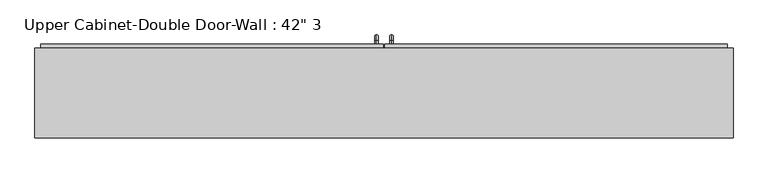
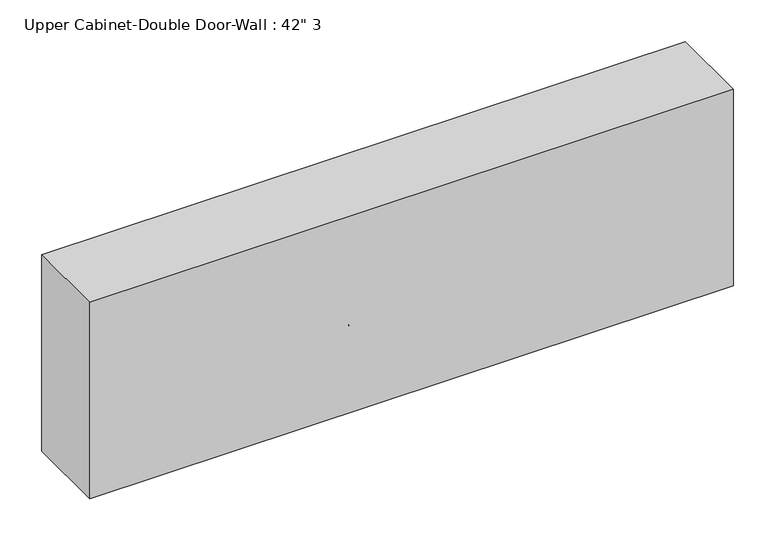
"""IFC4 building model written with IfcOpenShell, lengths in millimetres: furniture geometry."""

from ifc_helpers import new_model, si_unit, point, frame, origin, place, context, project, spatial, polyline, circle_curve, ellipse_curve, trimmed, outline, extrude, faceted_brep, source, transform, mapped, element, save
from ifc_brep_helpers import plane_surface, cylinder_surface, revolved_surface, advanced_brep


def furniture_a4bc473d(model_context):
    return source(origin(), model_context, "Body", "SolidModel", [
        extrude(outline(polyline([(32.9461628, 374.65), (1191.8211628, 374.65), (1191.8211628, 342.9), (32.9461628, 342.9), (32.9461628, 374.65)])), frame((0.0, 0.0, 1390.65), z_axis=(0.0, 0.0, 1.0), x_axis=(1.0, 0.0, 0.0)), (0.0, 0.0, 1.0), 723.9),
        extrude(outline(polyline([(-1132.2788372, 374.65), (26.5961628, 374.65), (26.5961628, 342.9), (-1132.2788372, 342.9), (-1132.2788372, 374.65)])), frame((0.0, 0.0, 1390.65), z_axis=(0.0, 0.0, 1.0), x_axis=(1.0, 0.0, 0.0)), (0.0, 0.0, 1.0), 723.9),
        advanced_brep(
        [(4.3711628, 374.65, 1517.65), (4.3711628, 374.65, 1530.35), (4.3711628, 387.35, 1517.65), (4.3711628, 387.35, 1530.35), (4.3711628, 406.4, 1511.3), (4.3711628, 393.7, 1511.3), (4.3711628, 393.7, 1435.1), (4.3711628, 406.4, 1435.1), (4.3711628, 387.35, 1416.05), (4.3711628, 387.35, 1428.75), (4.3711628, 374.65, 1428.75), (4.3711628, 374.65, 1416.05)],
        [
            (0, 1, circle_curve(frame((4.3711628, 374.65, 1524.0), z_axis=(0.0, -1.0, 0.0), x_axis=(0.0, 0.0, 1.0)), 6.35)),
            (1, 0, circle_curve(frame((4.3711628, 374.65, 1524.0), z_axis=(0.0, -1.0, 0.0), x_axis=(0.0, 0.0, 1.0)), 6.35)),
            (0, 2),
            (2, 3, circle_curve(frame((4.3711628, 387.35, 1524.0), z_axis=(0.0, -1.0, 0.0), x_axis=(0.0, 0.0, 1.0)), 6.35)),
            (3, 1),
            (3, 2, circle_curve(frame((4.3711628, 387.35, 1524.0), z_axis=(0.0, -1.0, 0.0), x_axis=(0.0, 0.0, 1.0)), 6.35)),
            (4, 3, circle_curve(frame((4.3711628, 387.35, 1511.3), z_axis=(1.0, 0.0, 0.0), x_axis=(0.0, 0.0, 1.0)), 19.05)),
            (2, 5, circle_curve(frame((4.3711628, 387.35, 1511.3), z_axis=(-1.0, 0.0, 0.0), x_axis=(0.0, 0.0, 1.0)), 6.35)),
            (5, 4, circle_curve(frame((4.3711628, 400.05, 1511.3), z_axis=(0.0, 0.0, 1.0), x_axis=(0.0, 1.0, 0.0)), 6.35)),
            (4, 5, circle_curve(frame((4.3711628, 400.05, 1511.3), z_axis=(0.0, 0.0, 1.0), x_axis=(0.0, 1.0, 0.0)), 6.35)),
            (5, 6),
            (6, 7, circle_curve(frame((4.3711628, 400.05, 1435.1), z_axis=(0.0, 0.0, 1.0), x_axis=(0.0, 1.0, 0.0)), 6.35)),
            (7, 4),
            (7, 6, circle_curve(frame((4.3711628, 400.05, 1435.1), z_axis=(0.0, 0.0, 1.0), x_axis=(0.0, 1.0, 0.0)), 6.35)),
            (8, 7, circle_curve(frame((4.3711628, 387.35, 1435.1), z_axis=(1.0, 0.0, 0.0), x_axis=(0.0, 1.0, 0.0)), 19.05)),
            (6, 9, circle_curve(frame((4.3711628, 387.35, 1435.1), z_axis=(-1.0, 0.0, 0.0), x_axis=(0.0, 1.0, 0.0)), 6.35)),
            (9, 8, circle_curve(frame((4.3711628, 387.35, 1422.4), z_axis=(0.0, 1.0, 0.0), x_axis=(0.0, 0.0, -1.0)), 6.35)),
            (8, 9, circle_curve(frame((4.3711628, 387.35, 1422.4), z_axis=(0.0, 1.0, 0.0), x_axis=(0.0, 0.0, -1.0)), 6.35)),
            (10, 11, circle_curve(frame((4.3711628, 374.65, 1422.4), z_axis=(0.0, -1.0, 0.0), x_axis=(0.0, 0.0, -1.0)), 6.35)),
            (11, 10, circle_curve(frame((4.3711628, 374.65, 1422.4), z_axis=(0.0, -1.0, 0.0), x_axis=(0.0, 0.0, -1.0)), 6.35)),
            (9, 10),
            (11, 8),
        ],
        [
            plane_surface(frame((-1.9788372, 374.65, 1524.0), z_axis=(0.0, -1.0, 0.0), x_axis=(0.0, 0.0, 1.0))),
            cylinder_surface(frame((4.3711628, 374.65, 1524.0), z_axis=(0.0, -1.0, 0.0), x_axis=(0.0, 0.0, 1.0)), 6.35),
            revolved_surface(trimmed(ellipse_curve(frame((4.3711628, 387.35, 1524.0), z_axis=(0.0, -1.0, 0.0), x_axis=(0.0, 0.0, 1.0)), 6.35, 6.35), [point((4.3711628, 387.35, 1517.65))], [point((4.3711628, 387.35, 1530.35))], True, "CARTESIAN"), (4.3711628, 387.35, 1511.3), (-1.0, 0.0, 0.0)),
            revolved_surface(trimmed(ellipse_curve(frame((4.3711628, 387.35, 1524.0), z_axis=(0.0, -1.0, 0.0), x_axis=(0.0, 0.0, 1.0)), 6.35, 6.35), [point((4.3711628, 387.35, 1530.35))], [point((4.3711628, 387.35, 1517.65))], True, "CARTESIAN"), (4.3711628, 387.35, 1511.3), (-1.0, 0.0, 0.0)),
            cylinder_surface(frame((4.3711628, 400.05, 1511.3), z_axis=(0.0, 0.0, 1.0), x_axis=(0.0, 1.0, 0.0)), 6.35),
            revolved_surface(trimmed(ellipse_curve(frame((4.3711628, 400.05, 1435.1), z_axis=(0.0, 0.0, 1.0), x_axis=(0.0, 1.0, 0.0)), 6.35, 6.35), [point((4.3711628, 393.7, 1435.1))], [point((4.3711628, 406.4, 1435.1))], True, "CARTESIAN"), (4.3711628, 387.35, 1435.1), (-1.0, 0.0, 0.0)),
            revolved_surface(trimmed(ellipse_curve(frame((4.3711628, 400.05, 1435.1), z_axis=(0.0, 0.0, 1.0), x_axis=(0.0, 1.0, 0.0)), 6.35, 6.35), [point((4.3711628, 406.4, 1435.1))], [point((4.3711628, 393.7, 1435.1))], True, "CARTESIAN"), (4.3711628, 387.35, 1435.1), (-1.0, 0.0, 0.0)),
            plane_surface(frame((-1.9788372, 374.65, 1422.4), z_axis=(0.0, -1.0, 0.0), x_axis=(0.0, 0.0, -1.0))),
            cylinder_surface(frame((4.3711628, 387.35, 1422.4), z_axis=(0.0, 1.0, 0.0), x_axis=(0.0, 0.0, -1.0)), 6.35),
        ],
        [
            (0, [[1, 2]]),
            (1, [[-1, 3, 4, 5]]),
            (1, [[-2, -5, 6, -3]]),
            (2, [[7, -4, 8, 9]]),
            (3, [[-8, -6, -7, 10]]),
            (4, [[-9, 11, 12, 13]]),
            (4, [[-10, -13, 14, -11]]),
            (5, [[15, -12, 16, 17]]),
            (6, [[-16, -14, -15, 18]]),
            (7, [[19, 20]]),
            (8, [[-17, 21, -20, 22]]),
            (8, [[-18, -22, -19, -21]]),
        ],
    ),
        advanced_brep(
        [(55.1711628, 374.65, 1517.65), (55.1711628, 374.65, 1530.35), (55.1711628, 387.35, 1517.65), (55.1711628, 387.35, 1530.35), (55.1711628, 406.4, 1511.3), (55.1711628, 393.7, 1511.3), (55.1711628, 393.7, 1435.1), (55.1711628, 406.4, 1435.1), (55.1711628, 387.35, 1416.05), (55.1711628, 387.35, 1428.75), (55.1711628, 374.65, 1428.75), (55.1711628, 374.65, 1416.05)],
        [
            (0, 1, circle_curve(frame((55.1711628, 374.65, 1524.0), z_axis=(0.0, -1.0, 0.0), x_axis=(0.0, 0.0, -1.0)), 6.35)),
            (1, 0, circle_curve(frame((55.1711628, 374.65, 1524.0), z_axis=(0.0, -1.0, 0.0), x_axis=(0.0, 0.0, -1.0)), 6.35)),
            (0, 2),
            (2, 3, circle_curve(frame((55.1711628, 387.35, 1524.0), z_axis=(0.0, -1.0, 0.0), x_axis=(0.0, 0.0, -1.0)), 6.35)),
            (3, 1),
            (3, 2, circle_curve(frame((55.1711628, 387.35, 1524.0), z_axis=(0.0, -1.0, 0.0), x_axis=(0.0, 0.0, -1.0)), 6.35)),
            (4, 3, circle_curve(frame((55.1711628, 387.35, 1511.3), z_axis=(1.0, 0.0, 0.0), x_axis=(0.0, 0.0, 1.0)), 19.05)),
            (2, 5, circle_curve(frame((55.1711628, 387.35, 1511.3), z_axis=(-1.0, 0.0, 0.0), x_axis=(0.0, 0.0, 1.0)), 6.35)),
            (5, 4, circle_curve(frame((55.1711628, 400.05, 1511.3), z_axis=(0.0, 0.0, 1.0), x_axis=(0.0, -1.0, 0.0)), 6.35)),
            (4, 5, circle_curve(frame((55.1711628, 400.05, 1511.3), z_axis=(0.0, 0.0, 1.0), x_axis=(0.0, -1.0, 0.0)), 6.35)),
            (5, 6),
            (6, 7, circle_curve(frame((55.1711628, 400.05, 1435.1), z_axis=(0.0, 0.0, 1.0), x_axis=(0.0, -1.0, 0.0)), 6.35)),
            (7, 4),
            (7, 6, circle_curve(frame((55.1711628, 400.05, 1435.1), z_axis=(0.0, 0.0, 1.0), x_axis=(0.0, -1.0, 0.0)), 6.35)),
            (8, 7, circle_curve(frame((55.1711628, 387.35, 1435.1), z_axis=(1.0, 0.0, 0.0), x_axis=(0.0, 1.0, 0.0)), 19.05)),
            (6, 9, circle_curve(frame((55.1711628, 387.35, 1435.1), z_axis=(-1.0, 0.0, 0.0), x_axis=(0.0, 1.0, 0.0)), 6.35)),
            (9, 8, circle_curve(frame((55.1711628, 387.35, 1422.4), z_axis=(0.0, 1.0, 0.0), x_axis=(0.0, 0.0, 1.0)), 6.35)),
            (8, 9, circle_curve(frame((55.1711628, 387.35, 1422.4), z_axis=(0.0, 1.0, 0.0), x_axis=(0.0, 0.0, 1.0)), 6.35)),
            (10, 11, circle_curve(frame((55.1711628, 374.65, 1422.4), z_axis=(0.0, -1.0, 0.0), x_axis=(0.0, 0.0, 1.0)), 6.35)),
            (11, 10, circle_curve(frame((55.1711628, 374.65, 1422.4), z_axis=(0.0, -1.0, 0.0), x_axis=(0.0, 0.0, 1.0)), 6.35)),
            (9, 10),
            (11, 8),
        ],
        [
            plane_surface(frame((48.8211628, 374.65, 1524.0), z_axis=(0.0, -1.0, 0.0), x_axis=(0.0, 0.0, 1.0))),
            cylinder_surface(frame((55.1711628, 374.65, 1524.0), z_axis=(0.0, -1.0, 0.0), x_axis=(0.0, 0.0, -1.0)), 6.35),
            revolved_surface(trimmed(ellipse_curve(frame((55.1711628, 387.35, 1524.0), z_axis=(0.0, -1.0, 0.0), x_axis=(0.0, 0.0, -1.0)), 6.35, 6.35), [point((55.1711628, 387.35, 1517.65))], [point((55.1711628, 387.35, 1530.35))], True, "CARTESIAN"), (55.1711628, 387.35, 1511.3), (-1.0, 0.0, 0.0)),
            revolved_surface(trimmed(ellipse_curve(frame((55.1711628, 387.35, 1524.0), z_axis=(0.0, -1.0, 0.0), x_axis=(0.0, 0.0, -1.0)), 6.35, 6.35), [point((55.1711628, 387.35, 1530.35))], [point((55.1711628, 387.35, 1517.65))], True, "CARTESIAN"), (55.1711628, 387.35, 1511.3), (-1.0, 0.0, 0.0)),
            cylinder_surface(frame((55.1711628, 400.05, 1511.3), z_axis=(0.0, 0.0, 1.0), x_axis=(0.0, -1.0, 0.0)), 6.35),
            revolved_surface(trimmed(ellipse_curve(frame((55.1711628, 400.05, 1435.1), z_axis=(0.0, 0.0, 1.0), x_axis=(0.0, -1.0, 0.0)), 6.35, 6.35), [point((55.1711628, 393.7, 1435.1))], [point((55.1711628, 406.4, 1435.1))], True, "CARTESIAN"), (55.1711628, 387.35, 1435.1), (-1.0, 0.0, 0.0)),
            revolved_surface(trimmed(ellipse_curve(frame((55.1711628, 400.05, 1435.1), z_axis=(0.0, 0.0, 1.0), x_axis=(0.0, -1.0, 0.0)), 6.35, 6.35), [point((55.1711628, 406.4, 1435.1))], [point((55.1711628, 393.7, 1435.1))], True, "CARTESIAN"), (55.1711628, 387.35, 1435.1), (-1.0, 0.0, 0.0)),
            plane_surface(frame((48.8211628, 374.65, 1422.4), z_axis=(0.0, -1.0, 0.0), x_axis=(0.0, 0.0, -1.0))),
            cylinder_surface(frame((55.1711628, 387.35, 1422.4), z_axis=(0.0, 1.0, 0.0), x_axis=(0.0, 0.0, 1.0)), 6.35),
        ],
        [
            (0, [[1, 2]]),
            (1, [[-1, 3, 4, 5]]),
            (1, [[-2, -5, 6, -3]]),
            (2, [[7, -4, 8, 9]]),
            (3, [[-8, -6, -7, 10]]),
            (4, [[-9, 11, 12, 13]]),
            (4, [[-10, -13, 14, -11]]),
            (5, [[15, -12, 16, 17]]),
            (6, [[-16, -14, -15, 18]]),
            (7, [[19, 20]]),
            (8, [[-17, 21, -20, 22]]),
            (8, [[-18, -22, -19, -21]]),
        ],
    ),
        faceted_brep([(-1151.3288372, 57.15, 2133.6), (-1151.3288372, 57.15, 1371.6), (1210.8711628, 57.15, 1371.6), (1210.8711628, 57.15, 2133.6), (-1151.3288372, 361.95, 2133.6), (1210.8711628, 361.95, 2133.6), (1210.8711628, 361.95, 1371.6), (-1151.3288372, 361.95, 1371.6), (-1132.2788372, 361.95, 2114.55), (-1132.2788372, 361.95, 1390.65), (1191.8211628, 361.95, 1390.65), (1191.8211628, 361.95, 2114.55), (1191.8211628, 76.2, 2114.55), (-1132.2788372, 76.2, 2114.55), (1191.8211628, 76.2, 1390.65), (-1132.2788372, 76.2, 1390.65)], [[[0, 1, 2, 3]], [[4, 5, 6, 7], [8, 9, 10, 11]], [[1, 0, 4, 7]], [[2, 1, 7, 6]], [[3, 2, 6, 5]], [[0, 3, 5, 4]], [[8, 11, 12, 13]], [[11, 10, 14, 12]], [[10, 9, 15, 14]], [[9, 8, 13, 15]], [[13, 12, 14, 15]]]),
    ])


if __name__ == "__main__":
    model = new_model("IFC4")
    model_context = context("Model", 3, world=origin())
    ifc_project = project(units=[si_unit("LENGTHUNIT", "METRE", prefix="MILLI")], contexts=[model_context])
    site = spatial("IfcSite", under=ifc_project)
    building = spatial("IfcBuilding", under=site)
    placement = place(None, origin())
    furniture_shape = furniture_a4bc473d(model_context)
    element("IfcFurniture", 1, ObjectType="Upper Cabinet-Double Door-Wall : 42\" 3", at=placement, inside=building, context=model_context, shape_type="MappedRepresentation", body=[
        mapped(furniture_shape, transform((0.0, 0.0, 0.0), x_axis=(1.0, 0.0, 0.0), y_axis=(0.0, 1.0, 0.0), z_axis=(0.0, 0.0, 1.0))),
    ])
    save(model, "model.ifc")

# Revit data of these elements
# Type "Upper Cabinet-Double Door-Wall : 42\" 3"
#   Assembly Code = "C1030410"
#   Depth = 1' - 0"
#   Height = 2' - 6"
#   Top Of Cabinet = 7' - 0"
#   Width = 7' - 9"
#   Cabinet Material = none
#   Door/Drawer Material = none
#   Handle Material = Cabinets - Handles
#   Default Elevation = 0
# Element 1 (IfcFurniture, "Upper Cabinet-Double Door-Wall : 42\" 3")
#   Materials on its faces: "Cabinets - Handles", "Cabinet"
# Materials
#   "Cabinets - Handles": colour RGB 57 57 57, transparency 0
#   "Cabinet": colour RGB 204 122 2, transparency 0
